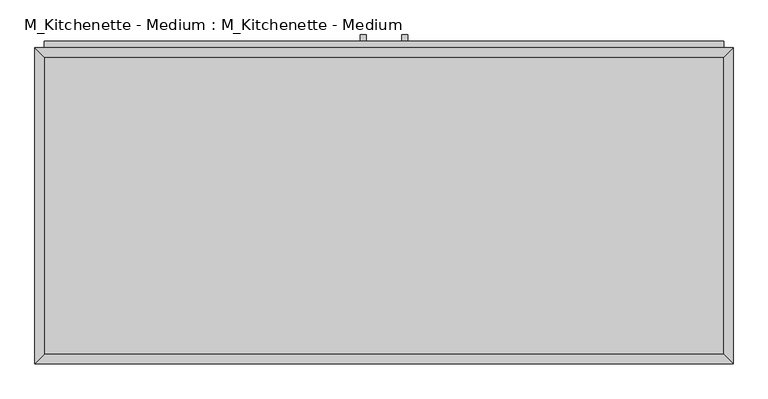
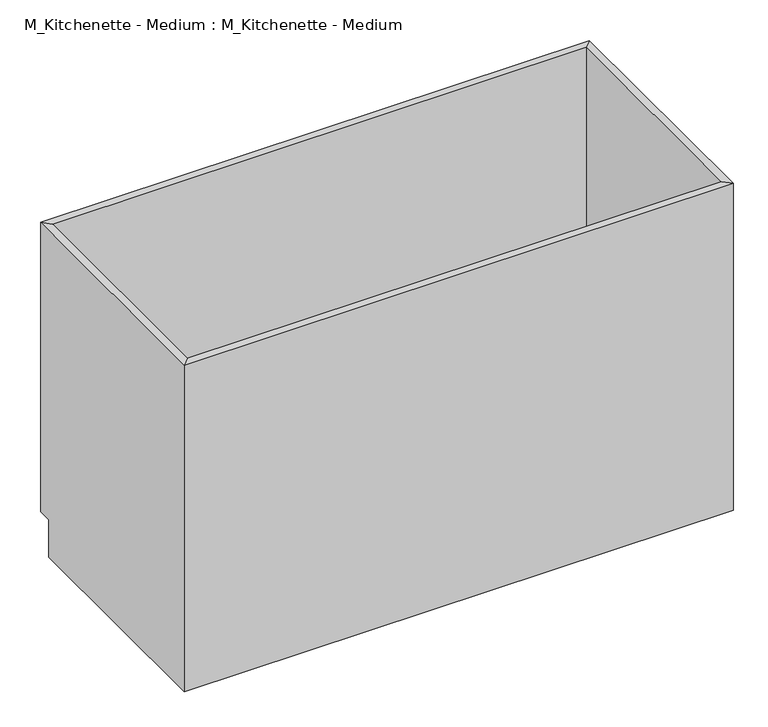
"""IFC4 building model written with IfcOpenShell, lengths in millimetres: proxy geometry, M_Kitchenette - Medium : M_Kitchenette - Medium."""

from ifc_helpers import new_model, si_unit, frame, origin, place, context, project, spatial, polyline, outline, extrude, faceted_brep, source, transform, mapped, element, save


def m_kitchenette_medium_m_kitchenette_medium_71e50c56(model_context):
    return source(origin(), model_context, "Body", "SolidModel", [
        extrude(outline(polyline([(694.6877049, 19.05), (-657.2122951, 19.05), (-657.2122951, 610.95), (694.6877049, 610.95), (694.6877049, 19.05)])), frame((0.0, 0.0, 100.0), z_axis=(0.0, 0.0, 1.0), x_axis=(1.0, 0.0, 0.0)), (0.0, 0.0, 1.0), 19.05),
        extrude(outline(polyline([(-16.1872951, 655.4), (-16.1872951, 642.7), (-28.8872951, 642.7), (-28.8872951, 655.4), (-16.1872951, 655.4)])), frame((0.0, 0.0, 595.6), z_axis=(0.0, 0.0, 1.0), x_axis=(1.0, 0.0, 0.0)), (0.0, 0.0, 1.0), 101.6),
        extrude(outline(polyline([(66.3627049, 655.4), (66.3627049, 642.7), (53.6627049, 642.7), (53.6627049, 655.4), (66.3627049, 655.4)])), frame((0.0, 0.0, 595.6), z_axis=(0.0, 0.0, 1.0), x_axis=(1.0, 0.0, 0.0)), (0.0, 0.0, 1.0), 101.6),
        faceted_brep([(694.6877049, 610.95, 875.0), (-657.2122951, 610.95, 875.0), (-657.2122951, 610.95, 100.0), (694.6877049, 610.95, 100.0), (713.7377049, 630.0, 875.0), (-676.2622951, 630.0, 875.0), (713.7377049, 630.0, 100.0), (-676.2622951, 630.0, 100.0), (-657.2122951, 19.05, 875.0), (-657.2122951, 19.05, 100.0), (-657.2122951, 595.0, 100.0), (-676.2622951, 0.0, 875.0), (-676.2622951, 595.0, 100.0), (-676.2622951, 595.0, 0.0), (-676.2622951, 0.0, 0.0), (694.6877049, 19.05, 875.0), (694.6877049, 19.05, 100.0), (713.7377049, 0.0, 875.0), (713.7377049, 0.0, 0.0), (694.6877049, 595.0, 100.0), (713.7377049, 595.0, 0.0), (713.7377049, 595.0, 100.0)], [[[0, 1, 2, 3]], [[0, 4, 5, 1]], [[4, 6, 7, 5]], [[2, 7, 6, 3]], [[1, 8, 9, 10, 2]], [[5, 11, 8, 1]], [[7, 12, 13, 14, 11, 5]], [[2, 10, 12, 7]], [[8, 15, 16, 9]], [[11, 17, 15, 8]], [[14, 18, 17, 11]], [[3, 19, 16, 15, 0]], [[0, 15, 17, 4]], [[4, 17, 18, 20, 21, 6]], [[6, 21, 19, 3]], [[10, 9, 16, 19]], [[18, 14, 13, 20]], [[13, 12, 10, 19, 21, 20]]]),
        extrude(outline(polyline([(9.2127049, 642.7), (9.2127049, 630.0), (-657.2122951, 630.0), (-657.2122951, 642.7), (9.2127049, 642.7)])), frame((0.0, 0.0, 119.05), z_axis=(0.0, 0.0, 1.0), x_axis=(1.0, 0.0, 0.0)), (0.0, 0.0, 1.0), 616.25),
        extrude(outline(polyline([(694.6877049, 642.7), (694.6877049, 630.0), (28.2627049, 630.0), (28.2627049, 642.7), (694.6877049, 642.7)])), frame((0.0, 0.0, 119.05), z_axis=(0.0, 0.0, 1.0), x_axis=(1.0, 0.0, 0.0)), (0.0, 0.0, 1.0), 616.25),
        extrude(outline(polyline([(694.6877049, 642.7), (694.6877049, 630.0), (-657.2122951, 630.0), (-657.2122951, 642.7), (694.6877049, 642.7)])), frame((0.0, 0.0, 754.35), z_axis=(0.0, 0.0, 1.0), x_axis=(1.0, 0.0, 0.0)), (0.0, 0.0, 1.0), 101.6),
    ])


if __name__ == "__main__":
    model = new_model("IFC4")
    model_context = context("Model", 3, world=origin())
    ifc_project = project(units=[si_unit("LENGTHUNIT", "METRE", prefix="MILLI")], contexts=[model_context])
    site = spatial("IfcSite", under=ifc_project)
    building = spatial("IfcBuilding", under=site)
    placement = place(None, origin())
    m_kitchenette_medium_m_kitchenette_medium_shape = m_kitchenette_medium_m_kitchenette_medium_71e50c56(model_context)
    element("IfcBuildingElementProxy", 1, Name="M_Kitchenette - Medium : M_Kitchenette - Medium", ObjectType="M_Kitchenette - Medium : M_Kitchenette - Medium", at=placement, inside=building, context=model_context, shape_type="MappedRepresentation", body=[
        mapped(m_kitchenette_medium_m_kitchenette_medium_shape, transform((0.0, 0.0, 0.0), x_axis=(1.0, 0.0, 0.0), y_axis=(0.0, 1.0, 0.0), z_axis=(0.0, 0.0, 1.0))),
    ])
    save(model, "model.ifc")

# Revit data of these elements
# Type "M_Kitchenette - Medium : M_Kitchenette - Medium"
#   Sink Opening Depth = 1.148294 ft
#   Sink Location To Wall = 0.492126 ft
#   Sink Location = 3.28084 ft
#   Counter Thickness = 0.131234 ft
#   Counter Length = 6.56168 ft
#   Cabinet Width = 4.560367 ft
#   Cabinet Height = 2.870735 ft
#   Cabinet Depth = 2.066929 ft
#   Toe Depth = 0.114829 ft
#   Toe Height = 0.328084 ft
#   Cabinet Material = Cabinets
#   Door/Drawer Material = Cabinets
#   Handle Material = Cabinets - Handles
#   Default Elevation = 0
# Element 1 (IfcBuildingElementProxy, "M_Kitchenette - Medium : M_Kitchenette - Medium")
#   Materials on its faces: "Cabinets", "Cabinets - Handles"
# Materials
#   "Cabinets": colour RGB 249 249 249, transparency 0
#   "Cabinets - Handles": class "Metal", colour RGB 57 57 57, transparency 0
